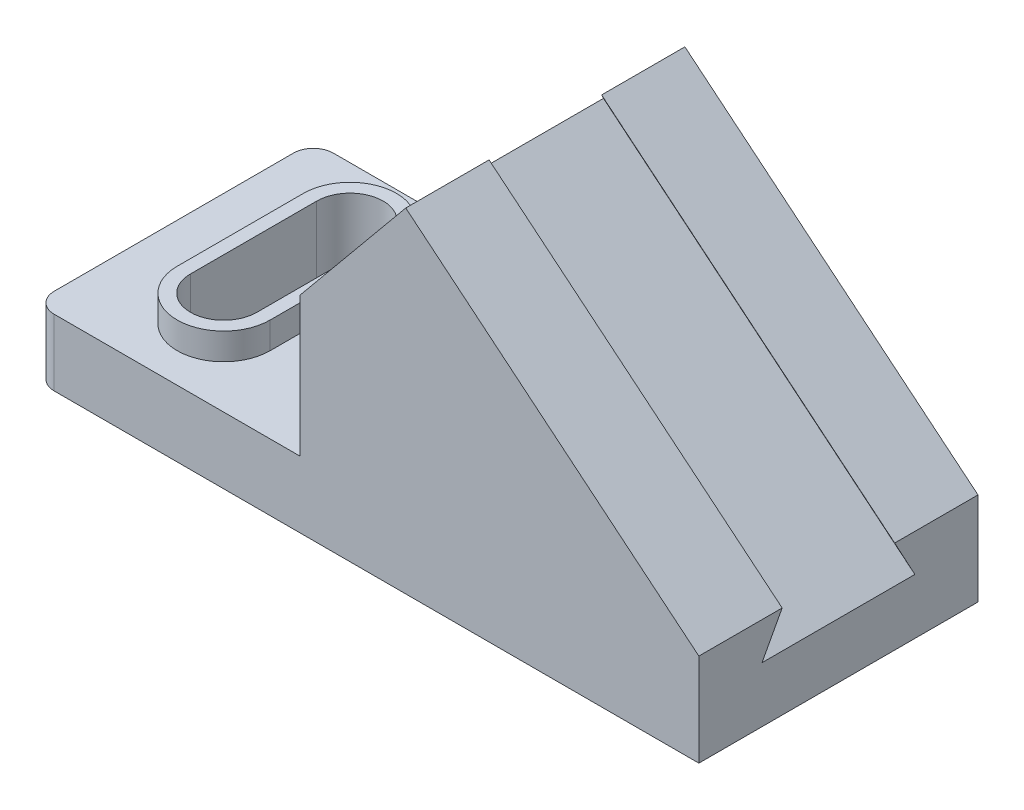
ISO-10303-21;
HEADER;
FILE_DESCRIPTION(('STEP AP214'),'2;1');
FILE_NAME('part.step','',(''),(''),'','','');
FILE_SCHEMA(('AUTOMOTIVE_DESIGN { 1 0 10303 214 1 1 1 1 }'));
ENDSEC;
DATA;
#1=APPLICATION_CONTEXT('core data for automotive mechanical design processes');
#2=APPLICATION_PROTOCOL_DEFINITION('international standard','automotive_design',2000,#1);
#3=PRODUCT_CONTEXT('',#1,'mechanical');
#4=PRODUCT('Part','Part','',(#3));
#5=PRODUCT_RELATED_PRODUCT_CATEGORY('part','',(#4));
#6=PRODUCT_DEFINITION_FORMATION('','',#4);
#7=PRODUCT_DEFINITION_CONTEXT('part definition',#1,'design');
#8=PRODUCT_DEFINITION('design','',#6,#7);
#9=PRODUCT_DEFINITION_SHAPE('','',#8);
#10=(LENGTH_UNIT() NAMED_UNIT(*) SI_UNIT(.MILLI.,.METRE.));
#11=(NAMED_UNIT(*) PLANE_ANGLE_UNIT() SI_UNIT($,.RADIAN.));
#12=(NAMED_UNIT(*) SI_UNIT($,.STERADIAN.) SOLID_ANGLE_UNIT());
#13=UNCERTAINTY_MEASURE_WITH_UNIT(LENGTH_MEASURE(1.E-05),#10,'distance_accuracy_value','');
#14=(GEOMETRIC_REPRESENTATION_CONTEXT(3) GLOBAL_UNCERTAINTY_ASSIGNED_CONTEXT((#13)) GLOBAL_UNIT_ASSIGNED_CONTEXT((#10,
#11,#12)) REPRESENTATION_CONTEXT('',''));
#15=CARTESIAN_POINT('',(0.,0.,0.));
#16=DIRECTION('',(0.,0.,1.));
#17=DIRECTION('',(1.,0.,0.));
#18=AXIS2_PLACEMENT_3D('',#15,#16,#17);
#19=CARTESIAN_POINT('',(-100.,9.99999999999999,21.));
#20=DIRECTION('',(0.,-1.,0.));
#21=DIRECTION('',(0.,0.,-1.));
#22=AXIS2_PLACEMENT_3D('',#19,#20,#21);
#23=PLANE('',#22);
#24=DIRECTION('',(-1.,0.,0.));
#25=VECTOR('',#24,1.);
#26=CARTESIAN_POINT('',(-100.,9.99999999999999,-21.));
#27=LINE('',#26,#25);
#28=CARTESIAN_POINT('',(-60.,9.99999999999999,-21.));
#29=VERTEX_POINT('',#28);
#30=CARTESIAN_POINT('',(-97.,9.99999999999999,-21.));
#31=VERTEX_POINT('',#30);
#32=EDGE_CURVE('E213',#29,#31,#27,.T.);
#33=ORIENTED_EDGE('',*,*,#32,.T.);
#34=CARTESIAN_POINT('',(-97.,9.99999999999999,-18.));
#35=DIRECTION('',(0.,-1.,0.));
#36=DIRECTION('',(0.,0.,-1.));
#37=AXIS2_PLACEMENT_3D('',#34,#35,#36);
#38=CIRCLE('',#37,3.);
#39=CARTESIAN_POINT('',(-100.,9.99999999999999,-18.));
#40=VERTEX_POINT('',#39);
#41=EDGE_CURVE('E50',#31,#40,#38,.F.);
#42=ORIENTED_EDGE('',*,*,#41,.T.);
#43=DIRECTION('',(0.,0.,-1.));
#44=VECTOR('',#43,1.);
#45=CARTESIAN_POINT('',(-100.,9.99999999999999,21.));
#46=LINE('',#45,#44);
#47=CARTESIAN_POINT('',(-100.,9.99999999999999,18.));
#48=VERTEX_POINT('',#47);
#49=EDGE_CURVE('E235',#48,#40,#46,.T.);
#50=ORIENTED_EDGE('',*,*,#49,.F.);
#51=CARTESIAN_POINT('',(-97.,9.99999999999999,18.));
#52=DIRECTION('',(0.,-1.,0.));
#53=DIRECTION('',(0.,0.,-1.));
#54=AXIS2_PLACEMENT_3D('',#51,#52,#53);
#55=CIRCLE('',#54,3.);
#56=CARTESIAN_POINT('',(-97.,9.99999999999999,21.));
#57=VERTEX_POINT('',#56);
#58=EDGE_CURVE('E53',#48,#57,#55,.F.);
#59=ORIENTED_EDGE('',*,*,#58,.T.);
#60=DIRECTION('',(-1.,0.,0.));
#61=VECTOR('',#60,1.);
#62=CARTESIAN_POINT('',(-100.,9.99999999999999,21.));
#63=LINE('',#62,#61);
#64=CARTESIAN_POINT('',(-60.,9.99999999999999,21.));
#65=VERTEX_POINT('',#64);
#66=EDGE_CURVE('E288',#65,#57,#63,.T.);
#67=ORIENTED_EDGE('',*,*,#66,.F.);
#68=DIRECTION('',(0.,0.,-1.));
#69=VECTOR('',#68,1.);
#70=CARTESIAN_POINT('',(-60.,9.99999999999999,21.));
#71=LINE('',#70,#69);
#72=EDGE_CURVE('E232',#65,#29,#71,.T.);
#73=ORIENTED_EDGE('',*,*,#72,.T.);
#74=EDGE_LOOP('',(#33,#42,#50,#59,#67,#73));
#75=FACE_BOUND('',#74,.T.);
#76=CARTESIAN_POINT('',(-83.,9.99999999999999,-9.5));
#77=DIRECTION('',(0.,1.,0.));
#78=DIRECTION('',(0.,0.,1.));
#79=AXIS2_PLACEMENT_3D('',#76,#77,#78);
#80=CIRCLE('',#79,7.00000000000001);
#81=CARTESIAN_POINT('',(-76.,9.99999999999999,-9.5));
#82=VERTEX_POINT('',#81);
#83=CARTESIAN_POINT('',(-90.,9.99999999999999,-9.5));
#84=VERTEX_POINT('',#83);
#85=EDGE_CURVE('E317',#82,#84,#80,.T.);
#86=ORIENTED_EDGE('',*,*,#85,.F.);
#87=DIRECTION('',(0.,0.,-1.));
#88=VECTOR('',#87,1.);
#89=CARTESIAN_POINT('',(-76.,9.99999999999999,-9.5));
#90=LINE('',#89,#88);
#91=CARTESIAN_POINT('',(-76.,9.99999999999999,9.5));
#92=VERTEX_POINT('',#91);
#93=EDGE_CURVE('E306',#92,#82,#90,.T.);
#94=ORIENTED_EDGE('',*,*,#93,.F.);
#95=CARTESIAN_POINT('',(-83.,9.99999999999999,9.5));
#96=DIRECTION('',(0.,1.,0.));
#97=DIRECTION('',(0.,0.,1.));
#98=AXIS2_PLACEMENT_3D('',#95,#96,#97);
#99=CIRCLE('',#98,7.00000000000001);
#100=CARTESIAN_POINT('',(-90.,9.99999999999999,9.5));
#101=VERTEX_POINT('',#100);
#102=EDGE_CURVE('E309',#101,#92,#99,.T.);
#103=ORIENTED_EDGE('',*,*,#102,.F.);
#104=DIRECTION('',(0.,0.,1.));
#105=VECTOR('',#104,1.);
#106=CARTESIAN_POINT('',(-90.,9.99999999999999,-9.5));
#107=LINE('',#106,#105);
#108=EDGE_CURVE('E312',#84,#101,#107,.T.);
#109=ORIENTED_EDGE('',*,*,#108,.F.);
#110=EDGE_LOOP('',(#86,#94,#103,#109));
#111=FACE_BOUND('',#110,.T.);
#112=ADVANCED_FACE('F39',(#75,#111),#23,.F.);
#113=CARTESIAN_POINT('',(0.,22.7360288756917,21.));
#114=DIRECTION('',(-1.,0.,0.));
#115=DIRECTION('',(0.,-1.,0.));
#116=AXIS2_PLACEMENT_3D('',#113,#114,#115);
#117=PLANE('',#116);
#118=DIRECTION('',(0.,0.879756327177352,-0.475424867661984));
#119=VECTOR('',#118,1.);
#120=CARTESIAN_POINT('',(0.,15.5093629916643,7.62731912376527));
#121=LINE('',#120,#119);
#122=CARTESIAN_POINT('',(0.,8.34310868788543,11.5));
#123=VERTEX_POINT('',#122);
#124=CARTESIAN_POINT('',(-1.08873334261842E-13,13.9569215437046,8.4662665085682));
#125=VERTEX_POINT('',#124);
#126=EDGE_CURVE('E344',#123,#125,#121,.T.);
#127=ORIENTED_EDGE('',*,*,#126,.T.);
#128=DIRECTION('',(0.,0.,1.));
#129=VECTOR('',#128,1.);
#130=CARTESIAN_POINT('',(0.,13.9569215437045,21.));
#131=LINE('',#130,#129);
#132=CARTESIAN_POINT('',(0.,13.9569215437045,21.));
#133=VERTEX_POINT('',#132);
#134=EDGE_CURVE('E347',#125,#133,#131,.T.);
#135=ORIENTED_EDGE('',*,*,#134,.T.);
#136=DIRECTION('',(0.,1.,0.));
#137=VECTOR('',#136,1.);
#138=CARTESIAN_POINT('',(0.,22.7360288756917,21.));
#139=LINE('',#138,#137);
#140=CARTESIAN_POINT('',(0.,0.,21.));
#141=VERTEX_POINT('',#140);
#142=EDGE_CURVE('E225',#141,#133,#139,.T.);
#143=ORIENTED_EDGE('',*,*,#142,.F.);
#144=DIRECTION('',(0.,0.,-1.));
#145=VECTOR('',#144,1.);
#146=CARTESIAN_POINT('',(0.,0.,21.));
#147=LINE('',#146,#145);
#148=CARTESIAN_POINT('',(0.,0.,-21.));
#149=VERTEX_POINT('',#148);
#150=EDGE_CURVE('E221',#141,#149,#147,.T.);
#151=ORIENTED_EDGE('',*,*,#150,.T.);
#152=DIRECTION('',(0.,1.,0.));
#153=VECTOR('',#152,1.);
#154=CARTESIAN_POINT('',(0.,22.7360288756917,-21.));
#155=LINE('',#154,#153);
#156=CARTESIAN_POINT('',(0.,13.9569215437045,-21.));
#157=VERTEX_POINT('',#156);
#158=EDGE_CURVE('E214',#149,#157,#155,.T.);
#159=ORIENTED_EDGE('',*,*,#158,.T.);
#160=DIRECTION('',(0.,0.,1.));
#161=VECTOR('',#160,1.);
#162=CARTESIAN_POINT('',(0.,13.9569215437045,21.));
#163=LINE('',#162,#161);
#164=CARTESIAN_POINT('',(0.,13.9569215437045,-8.46626650856829));
#165=VERTEX_POINT('',#164);
#166=EDGE_CURVE('E194',#157,#165,#163,.T.);
#167=ORIENTED_EDGE('',*,*,#166,.T.);
#168=DIRECTION('',(0.,-0.879756327177356,-0.475424867661978));
#169=VECTOR('',#168,1.);
#170=CARTESIAN_POINT('',(0.,33.0762004794339,1.86589067747389));
#171=LINE('',#170,#169);
#172=CARTESIAN_POINT('',(0.,8.34310868788538,-11.5));
#173=VERTEX_POINT('',#172);
#174=EDGE_CURVE('E346',#165,#173,#171,.T.);
#175=ORIENTED_EDGE('',*,*,#174,.T.);
#176=DIRECTION('',(0.,0.,1.));
#177=VECTOR('',#176,1.);
#178=CARTESIAN_POINT('',(0.,8.34310868788541,21.));
#179=LINE('',#178,#177);
#180=EDGE_CURVE('E343',#173,#123,#179,.T.);
#181=ORIENTED_EDGE('',*,*,#180,.T.);
#182=EDGE_LOOP('',(#127,#135,#143,#151,#159,#167,#175,#181));
#183=FACE_BOUND('',#182,.T.);
#184=ADVANCED_FACE('F276',(#183),#117,.F.);
#185=CARTESIAN_POINT('',(-60.,31.,21.));
#186=DIRECTION('',(0.771778566555523,-0.635891377678218,0.));
#187=DIRECTION('',(0.635891377678218,0.771778566555523,0.));
#188=AXIS2_PLACEMENT_3D('',#185,#186,#187);
#189=PLANE('',#188);
#190=DIRECTION('',(0.,0.,-1.));
#191=VECTOR('',#190,1.);
#192=CARTESIAN_POINT('',(-44.1027155580446,50.2944641638881,21.));
#193=LINE('',#192,#191);
#194=CARTESIAN_POINT('',(-44.1027155580446,50.2944641638881,21.));
#195=VERTEX_POINT('',#194);
#196=CARTESIAN_POINT('',(-44.1027155580446,50.2944641638881,8.46626650856824));
#197=VERTEX_POINT('',#196);
#198=EDGE_CURVE('E239',#195,#197,#193,.T.);
#199=ORIENTED_EDGE('',*,*,#198,.T.);
#200=DIRECTION('',(0.520891721970854,0.632203990532382,-0.57357643635105));
#201=VECTOR('',#200,1.);
#202=CARTESIAN_POINT('',(-46.857791537814,46.9506405722212,11.5));
#203=LINE('',#202,#201);
#204=CARTESIAN_POINT('',(-46.857791537814,46.9506405722212,11.5));
#205=VERTEX_POINT('',#204);
#206=EDGE_CURVE('E357',#205,#197,#203,.T.);
#207=ORIENTED_EDGE('',*,*,#206,.F.);
#208=DIRECTION('',(0.,0.,1.));
#209=VECTOR('',#208,1.);
#210=CARTESIAN_POINT('',(-46.857791537814,46.9506405722212,-11.5));
#211=LINE('',#210,#209);
#212=CARTESIAN_POINT('',(-46.857791537814,46.9506405722212,-11.5));
#213=VERTEX_POINT('',#212);
#214=EDGE_CURVE('E364',#213,#205,#211,.T.);
#215=ORIENTED_EDGE('',*,*,#214,.F.);
#216=DIRECTION('',(-0.520891721970857,-0.632203990532386,-0.573576436351044));
#217=VECTOR('',#216,1.);
#218=CARTESIAN_POINT('',(-46.857791537814,46.9506405722212,-11.5));
#219=LINE('',#218,#217);
#220=CARTESIAN_POINT('',(-44.1027155580446,50.2944641638881,-8.46626650856829));
#221=VERTEX_POINT('',#220);
#222=EDGE_CURVE('E206',#221,#213,#219,.T.);
#223=ORIENTED_EDGE('',*,*,#222,.F.);
#224=DIRECTION('',(0.,0.,1.));
#225=VECTOR('',#224,1.);
#226=CARTESIAN_POINT('',(-44.1027155580446,50.2944641638881,-8.46626650856829));
#227=LINE('',#226,#225);
#228=CARTESIAN_POINT('',(-44.1027155580446,50.2944641638881,-21.));
#229=VERTEX_POINT('',#228);
#230=EDGE_CURVE('E188',#229,#221,#227,.T.);
#231=ORIENTED_EDGE('',*,*,#230,.F.);
#232=DIRECTION('',(-0.635891377678218,-0.771778566555523,0.));
#233=VECTOR('',#232,1.);
#234=CARTESIAN_POINT('',(-60.,31.,-21.));
#235=LINE('',#234,#233);
#236=CARTESIAN_POINT('',(-60.,31.,-21.));
#237=VERTEX_POINT('',#236);
#238=EDGE_CURVE('E205',#229,#237,#235,.T.);
#239=ORIENTED_EDGE('',*,*,#238,.T.);
#240=DIRECTION('',(0.,0.,-1.));
#241=VECTOR('',#240,1.);
#242=CARTESIAN_POINT('',(-60.,31.,21.));
#243=LINE('',#242,#241);
#244=CARTESIAN_POINT('',(-60.,31.,21.));
#245=VERTEX_POINT('',#244);
#246=EDGE_CURVE('E238',#245,#237,#243,.T.);
#247=ORIENTED_EDGE('',*,*,#246,.F.);
#248=DIRECTION('',(-0.635891377678218,-0.771778566555523,0.));
#249=VECTOR('',#248,1.);
#250=CARTESIAN_POINT('',(-60.,31.,21.));
#251=LINE('',#250,#249);
#252=EDGE_CURVE('E293',#195,#245,#251,.T.);
#253=ORIENTED_EDGE('',*,*,#252,.F.);
#254=EDGE_LOOP('',(#199,#207,#215,#223,#231,#239,#247,#253));
#255=FACE_BOUND('',#254,.T.);
#256=ADVANCED_FACE('F204',(#255),#189,.F.);
#257=CARTESIAN_POINT('',(-60.,9.99999999999999,21.));
#258=DIRECTION('',(1.,0.,0.));
#259=DIRECTION('',(0.,0.,-1.));
#260=AXIS2_PLACEMENT_3D('',#257,#258,#259);
#261=PLANE('',#260);
#262=DIRECTION('',(0.,-1.,0.));
#263=VECTOR('',#262,1.);
#264=CARTESIAN_POINT('',(-60.,9.99999999999999,-21.));
#265=LINE('',#264,#263);
#266=EDGE_CURVE('E215',#237,#29,#265,.T.);
#267=ORIENTED_EDGE('',*,*,#266,.T.);
#268=ORIENTED_EDGE('',*,*,#72,.F.);
#269=DIRECTION('',(0.,-1.,0.));
#270=VECTOR('',#269,1.);
#271=CARTESIAN_POINT('',(-60.,9.99999999999999,21.));
#272=LINE('',#271,#270);
#273=EDGE_CURVE('E289',#245,#65,#272,.T.);
#274=ORIENTED_EDGE('',*,*,#273,.F.);
#275=ORIENTED_EDGE('',*,*,#246,.T.);
#276=EDGE_LOOP('',(#267,#268,#274,#275));
#277=FACE_BOUND('',#276,.T.);
#278=ADVANCED_FACE('F381',(#277),#261,.F.);
#279=CARTESIAN_POINT('',(-100.,0.,21.));
#280=DIRECTION('',(1.,0.,0.));
#281=DIRECTION('',(0.,0.,-1.));
#282=AXIS2_PLACEMENT_3D('',#279,#280,#281);
#283=PLANE('',#282);
#284=ORIENTED_EDGE('',*,*,#49,.T.);
#285=DIRECTION('',(0.,-1.,0.));
#286=VECTOR('',#285,1.);
#287=CARTESIAN_POINT('',(-100.,0.,-18.));
#288=LINE('',#287,#286);
#289=CARTESIAN_POINT('',(-100.,0.,-18.));
#290=VERTEX_POINT('',#289);
#291=EDGE_CURVE('E260',#40,#290,#288,.T.);
#292=ORIENTED_EDGE('',*,*,#291,.T.);
#293=DIRECTION('',(0.,0.,-1.));
#294=VECTOR('',#293,1.);
#295=CARTESIAN_POINT('',(-100.,0.,21.));
#296=LINE('',#295,#294);
#297=CARTESIAN_POINT('',(-100.,0.,18.));
#298=VERTEX_POINT('',#297);
#299=EDGE_CURVE('E226',#298,#290,#296,.T.);
#300=ORIENTED_EDGE('',*,*,#299,.F.);
#301=DIRECTION('',(0.,-1.,0.));
#302=VECTOR('',#301,1.);
#303=CARTESIAN_POINT('',(-100.,0.,18.));
#304=LINE('',#303,#302);
#305=EDGE_CURVE('E253',#298,#48,#304,.F.);
#306=ORIENTED_EDGE('',*,*,#305,.T.);
#307=EDGE_LOOP('',(#284,#292,#300,#306));
#308=FACE_BOUND('',#307,.T.);
#309=ADVANCED_FACE('F266',(#308),#283,.F.);
#310=CARTESIAN_POINT('',(0.,0.,21.));
#311=DIRECTION('',(0.,1.,0.));
#312=DIRECTION('',(-1.,0.,0.));
#313=AXIS2_PLACEMENT_3D('',#310,#311,#312);
#314=PLANE('',#313);
#315=DIRECTION('',(0.,0.,-1.));
#316=VECTOR('',#315,1.);
#317=CARTESIAN_POINT('',(-78.,0.,20.9999999999999));
#318=LINE('',#317,#316);
#319=CARTESIAN_POINT('',(-78.,0.,9.5));
#320=VERTEX_POINT('',#319);
#321=CARTESIAN_POINT('',(-78.,0.,-9.5));
#322=VERTEX_POINT('',#321);
#323=EDGE_CURVE('E247',#320,#322,#318,.T.);
#324=ORIENTED_EDGE('',*,*,#323,.T.);
#325=CARTESIAN_POINT('',(-83.,0.,-9.5));
#326=DIRECTION('',(0.,1.,0.));
#327=DIRECTION('',(-1.,0.,0.));
#328=AXIS2_PLACEMENT_3D('',#325,#326,#327);
#329=CIRCLE('',#328,5.);
#330=CARTESIAN_POINT('',(-88.,0.,-9.5));
#331=VERTEX_POINT('',#330);
#332=EDGE_CURVE('E196',#322,#331,#329,.T.);
#333=ORIENTED_EDGE('',*,*,#332,.T.);
#334=DIRECTION('',(0.,0.,1.));
#335=VECTOR('',#334,1.);
#336=CARTESIAN_POINT('',(-88.,0.,21.));
#337=LINE('',#336,#335);
#338=CARTESIAN_POINT('',(-88.,0.,9.5));
#339=VERTEX_POINT('',#338);
#340=EDGE_CURVE('E245',#331,#339,#337,.T.);
#341=ORIENTED_EDGE('',*,*,#340,.T.);
#342=CARTESIAN_POINT('',(-83.,0.,9.5));
#343=DIRECTION('',(0.,1.,0.));
#344=DIRECTION('',(-1.,0.,0.));
#345=AXIS2_PLACEMENT_3D('',#342,#343,#344);
#346=CIRCLE('',#345,5.);
#347=EDGE_CURVE('E244',#339,#320,#346,.T.);
#348=ORIENTED_EDGE('',*,*,#347,.T.);
#349=EDGE_LOOP('',(#324,#333,#341,#348));
#350=FACE_BOUND('',#349,.T.);
#351=ORIENTED_EDGE('',*,*,#299,.T.);
#352=CARTESIAN_POINT('',(-97.,0.,-18.));
#353=DIRECTION('',(0.,1.,0.));
#354=DIRECTION('',(-1.,0.,0.));
#355=AXIS2_PLACEMENT_3D('',#352,#353,#354);
#356=CIRCLE('',#355,3.);
#357=CARTESIAN_POINT('',(-97.,0.,-21.));
#358=VERTEX_POINT('',#357);
#359=EDGE_CURVE('E265',#290,#358,#356,.F.);
#360=ORIENTED_EDGE('',*,*,#359,.T.);
#361=DIRECTION('',(1.,0.,0.));
#362=VECTOR('',#361,1.);
#363=CARTESIAN_POINT('',(0.,0.,-21.));
#364=LINE('',#363,#362);
#365=EDGE_CURVE('E224',#358,#149,#364,.T.);
#366=ORIENTED_EDGE('',*,*,#365,.T.);
#367=ORIENTED_EDGE('',*,*,#150,.F.);
#368=DIRECTION('',(1.,0.,0.));
#369=VECTOR('',#368,1.);
#370=CARTESIAN_POINT('',(0.,0.,21.));
#371=LINE('',#370,#369);
#372=CARTESIAN_POINT('',(-97.,0.,21.));
#373=VERTEX_POINT('',#372);
#374=EDGE_CURVE('E230',#373,#141,#371,.T.);
#375=ORIENTED_EDGE('',*,*,#374,.F.);
#376=CARTESIAN_POINT('',(-97.,0.,18.));
#377=DIRECTION('',(0.,1.,0.));
#378=DIRECTION('',(-1.,0.,0.));
#379=AXIS2_PLACEMENT_3D('',#376,#377,#378);
#380=CIRCLE('',#379,3.);
#381=EDGE_CURVE('E258',#373,#298,#380,.F.);
#382=ORIENTED_EDGE('',*,*,#381,.T.);
#383=EDGE_LOOP('',(#351,#360,#366,#367,#375,#382));
#384=FACE_BOUND('',#383,.T.);
#385=ADVANCED_FACE('F273',(#350,#384),#314,.F.);
#386=CARTESIAN_POINT('',(0.,0.,21.));
#387=DIRECTION('',(0.,0.,-1.));
#388=DIRECTION('',(-1.,0.,0.));
#389=AXIS2_PLACEMENT_3D('',#386,#387,#388);
#390=PLANE('',#389);
#391=ORIENTED_EDGE('',*,*,#66,.T.);
#392=DIRECTION('',(0.,-1.,0.));
#393=VECTOR('',#392,1.);
#394=CARTESIAN_POINT('',(-97.,0.,21.));
#395=LINE('',#394,#393);
#396=EDGE_CURVE('E11',#57,#373,#395,.T.);
#397=ORIENTED_EDGE('',*,*,#396,.T.);
#398=ORIENTED_EDGE('',*,*,#374,.T.);
#399=ORIENTED_EDGE('',*,*,#142,.T.);
#400=DIRECTION('',(-0.771778566555523,0.635891377678218,0.));
#401=VECTOR('',#400,1.);
#402=CARTESIAN_POINT('',(6.84960120406021,8.31333083654682,21.));
#403=LINE('',#402,#401);
#404=EDGE_CURVE('E200',#133,#195,#403,.T.);
#405=ORIENTED_EDGE('',*,*,#404,.T.);
#406=ORIENTED_EDGE('',*,*,#252,.T.);
#407=ORIENTED_EDGE('',*,*,#273,.T.);
#408=EDGE_LOOP('',(#391,#397,#398,#399,#405,#406,#407));
#409=FACE_BOUND('',#408,.T.);
#410=ADVANCED_FACE('F379',(#409),#390,.F.);
#411=CARTESIAN_POINT('',(0.,0.,-21.));
#412=DIRECTION('',(0.,0.,-1.));
#413=DIRECTION('',(-1.,0.,0.));
#414=AXIS2_PLACEMENT_3D('',#411,#412,#413);
#415=PLANE('',#414);
#416=ORIENTED_EDGE('',*,*,#365,.F.);
#417=DIRECTION('',(0.,-1.,0.));
#418=VECTOR('',#417,1.);
#419=CARTESIAN_POINT('',(-97.,9.99999999999999,-21.));
#420=LINE('',#419,#418);
#421=EDGE_CURVE('E65',#358,#31,#420,.F.);
#422=ORIENTED_EDGE('',*,*,#421,.T.);
#423=ORIENTED_EDGE('',*,*,#32,.F.);
#424=ORIENTED_EDGE('',*,*,#266,.F.);
#425=ORIENTED_EDGE('',*,*,#238,.F.);
#426=DIRECTION('',(-0.771778566555523,0.635891377678218,0.));
#427=VECTOR('',#426,1.);
#428=CARTESIAN_POINT('',(6.84960120406021,8.31333083654682,-21.));
#429=LINE('',#428,#427);
#430=EDGE_CURVE('E187',#157,#229,#429,.T.);
#431=ORIENTED_EDGE('',*,*,#430,.F.);
#432=ORIENTED_EDGE('',*,*,#158,.F.);
#433=EDGE_LOOP('',(#416,#422,#423,#424,#425,#431,#432));
#434=FACE_BOUND('',#433,.T.);
#435=ADVANCED_FACE('F212',(#434),#415,.T.);
#436=CARTESIAN_POINT('',(-83.,14.,-9.5));
#437=DIRECTION('',(0.,1.,0.));
#438=DIRECTION('',(0.,0.,1.));
#439=AXIS2_PLACEMENT_3D('',#436,#437,#438);
#440=PLANE('',#439);
#441=CARTESIAN_POINT('',(-83.,14.,-9.5));
#442=DIRECTION('',(0.,1.,0.));
#443=DIRECTION('',(0.,0.,1.));
#444=AXIS2_PLACEMENT_3D('',#441,#442,#443);
#445=CIRCLE('',#444,7.00000000000001);
#446=CARTESIAN_POINT('',(-76.,14.,-9.5));
#447=VERTEX_POINT('',#446);
#448=CARTESIAN_POINT('',(-90.,14.,-9.5));
#449=VERTEX_POINT('',#448);
#450=EDGE_CURVE('E307',#447,#449,#445,.T.);
#451=ORIENTED_EDGE('',*,*,#450,.T.);
#452=DIRECTION('',(0.,0.,1.));
#453=VECTOR('',#452,1.);
#454=CARTESIAN_POINT('',(-90.,14.,-9.5));
#455=LINE('',#454,#453);
#456=CARTESIAN_POINT('',(-90.,14.,9.5));
#457=VERTEX_POINT('',#456);
#458=EDGE_CURVE('E324',#449,#457,#455,.T.);
#459=ORIENTED_EDGE('',*,*,#458,.T.);
#460=CARTESIAN_POINT('',(-83.,14.,9.5));
#461=DIRECTION('',(0.,1.,0.));
#462=DIRECTION('',(0.,0.,1.));
#463=AXIS2_PLACEMENT_3D('',#460,#461,#462);
#464=CIRCLE('',#463,7.00000000000001);
#465=CARTESIAN_POINT('',(-76.,14.,9.5));
#466=VERTEX_POINT('',#465);
#467=EDGE_CURVE('E322',#457,#466,#464,.T.);
#468=ORIENTED_EDGE('',*,*,#467,.T.);
#469=DIRECTION('',(0.,0.,-1.));
#470=VECTOR('',#469,1.);
#471=CARTESIAN_POINT('',(-76.,14.,-9.5));
#472=LINE('',#471,#470);
#473=EDGE_CURVE('E304',#466,#447,#472,.T.);
#474=ORIENTED_EDGE('',*,*,#473,.T.);
#475=EDGE_LOOP('',(#451,#459,#468,#474));
#476=FACE_BOUND('',#475,.T.);
#477=DIRECTION('',(0.,0.,1.));
#478=VECTOR('',#477,1.);
#479=CARTESIAN_POINT('',(-88.,14.,-9.5));
#480=LINE('',#479,#478);
#481=CARTESIAN_POINT('',(-88.,14.,-9.5));
#482=VERTEX_POINT('',#481);
#483=CARTESIAN_POINT('',(-88.,14.,9.5));
#484=VERTEX_POINT('',#483);
#485=EDGE_CURVE('E339',#482,#484,#480,.T.);
#486=ORIENTED_EDGE('',*,*,#485,.F.);
#487=CARTESIAN_POINT('',(-83.,14.,-9.5));
#488=DIRECTION('',(0.,1.,0.));
#489=DIRECTION('',(0.,0.,1.));
#490=AXIS2_PLACEMENT_3D('',#487,#488,#489);
#491=CIRCLE('',#490,5.);
#492=CARTESIAN_POINT('',(-78.,14.,-9.5));
#493=VERTEX_POINT('',#492);
#494=EDGE_CURVE('E342',#493,#482,#491,.T.);
#495=ORIENTED_EDGE('',*,*,#494,.F.);
#496=DIRECTION('',(0.,0.,-1.));
#497=VECTOR('',#496,1.);
#498=CARTESIAN_POINT('',(-78.,14.,-9.5));
#499=LINE('',#498,#497);
#500=CARTESIAN_POINT('',(-78.,14.,9.5));
#501=VERTEX_POINT('',#500);
#502=EDGE_CURVE('E335',#501,#493,#499,.T.);
#503=ORIENTED_EDGE('',*,*,#502,.F.);
#504=CARTESIAN_POINT('',(-83.,14.,9.5));
#505=DIRECTION('',(0.,1.,0.));
#506=DIRECTION('',(0.,0.,1.));
#507=AXIS2_PLACEMENT_3D('',#504,#505,#506);
#508=CIRCLE('',#507,5.);
#509=EDGE_CURVE('E337',#484,#501,#508,.T.);
#510=ORIENTED_EDGE('',*,*,#509,.F.);
#511=EDGE_LOOP('',(#486,#495,#503,#510));
#512=FACE_BOUND('',#511,.T.);
#513=ADVANCED_FACE('F461',(#476,#512),#440,.T.);
#514=CARTESIAN_POINT('',(-83.,14.,-9.5));
#515=DIRECTION('',(0.,-1.,0.));
#516=DIRECTION('',(0.,0.,-1.));
#517=AXIS2_PLACEMENT_3D('',#514,#515,#516);
#518=CYLINDRICAL_SURFACE('',#517,7.00000000000001);
#519=ORIENTED_EDGE('',*,*,#85,.T.);
#520=DIRECTION('',(0.,-1.,0.));
#521=VECTOR('',#520,1.);
#522=CARTESIAN_POINT('',(-90.,14.,-9.5));
#523=LINE('',#522,#521);
#524=EDGE_CURVE('E220',#449,#84,#523,.T.);
#525=ORIENTED_EDGE('',*,*,#524,.F.);
#526=ORIENTED_EDGE('',*,*,#450,.F.);
#527=DIRECTION('',(0.,-1.,0.));
#528=VECTOR('',#527,1.);
#529=CARTESIAN_POINT('',(-76.,14.,-9.5));
#530=LINE('',#529,#528);
#531=EDGE_CURVE('E305',#447,#82,#530,.T.);
#532=ORIENTED_EDGE('',*,*,#531,.T.);
#533=EDGE_LOOP('',(#519,#525,#526,#532));
#534=FACE_BOUND('',#533,.T.);
#535=ADVANCED_FACE('F498',(#534),#518,.T.);
#536=CARTESIAN_POINT('',(-90.,14.,-9.5));
#537=DIRECTION('',(1.,0.,0.));
#538=DIRECTION('',(0.,0.,-1.));
#539=AXIS2_PLACEMENT_3D('',#536,#537,#538);
#540=PLANE('',#539);
#541=ORIENTED_EDGE('',*,*,#108,.T.);
#542=DIRECTION('',(0.,-1.,0.));
#543=VECTOR('',#542,1.);
#544=CARTESIAN_POINT('',(-90.,14.,9.5));
#545=LINE('',#544,#543);
#546=EDGE_CURVE('E298',#457,#101,#545,.T.);
#547=ORIENTED_EDGE('',*,*,#546,.F.);
#548=ORIENTED_EDGE('',*,*,#458,.F.);
#549=ORIENTED_EDGE('',*,*,#524,.T.);
#550=EDGE_LOOP('',(#541,#547,#548,#549));
#551=FACE_BOUND('',#550,.T.);
#552=ADVANCED_FACE('F510',(#551),#540,.F.);
#553=CARTESIAN_POINT('',(-83.,14.,9.5));
#554=DIRECTION('',(0.,-1.,0.));
#555=DIRECTION('',(0.,0.,-1.));
#556=AXIS2_PLACEMENT_3D('',#553,#554,#555);
#557=CYLINDRICAL_SURFACE('',#556,7.00000000000001);
#558=ORIENTED_EDGE('',*,*,#102,.T.);
#559=DIRECTION('',(0.,-1.,0.));
#560=VECTOR('',#559,1.);
#561=CARTESIAN_POINT('',(-76.,14.,9.5));
#562=LINE('',#561,#560);
#563=EDGE_CURVE('E299',#466,#92,#562,.T.);
#564=ORIENTED_EDGE('',*,*,#563,.F.);
#565=ORIENTED_EDGE('',*,*,#467,.F.);
#566=ORIENTED_EDGE('',*,*,#546,.T.);
#567=EDGE_LOOP('',(#558,#564,#565,#566));
#568=FACE_BOUND('',#567,.T.);
#569=ADVANCED_FACE('F517',(#568),#557,.T.);
#570=CARTESIAN_POINT('',(-76.,14.,-9.5));
#571=DIRECTION('',(-1.,0.,0.));
#572=DIRECTION('',(0.,0.,1.));
#573=AXIS2_PLACEMENT_3D('',#570,#571,#572);
#574=PLANE('',#573);
#575=ORIENTED_EDGE('',*,*,#93,.T.);
#576=ORIENTED_EDGE('',*,*,#531,.F.);
#577=ORIENTED_EDGE('',*,*,#473,.F.);
#578=ORIENTED_EDGE('',*,*,#563,.T.);
#579=EDGE_LOOP('',(#575,#576,#577,#578));
#580=FACE_BOUND('',#579,.T.);
#581=ADVANCED_FACE('F522',(#580),#574,.F.);
#582=CARTESIAN_POINT('',(-83.,14.,-9.5));
#583=DIRECTION('',(0.,-1.,0.));
#584=DIRECTION('',(0.,0.,-1.));
#585=AXIS2_PLACEMENT_3D('',#582,#583,#584);
#586=CYLINDRICAL_SURFACE('',#585,5.);
#587=DIRECTION('',(0.,-1.,0.));
#588=VECTOR('',#587,1.);
#589=CARTESIAN_POINT('',(-88.,14.,-9.5));
#590=LINE('',#589,#588);
#591=EDGE_CURVE('E316',#482,#331,#590,.T.);
#592=ORIENTED_EDGE('',*,*,#591,.T.);
#593=ORIENTED_EDGE('',*,*,#332,.F.);
#594=DIRECTION('',(0.,-1.,0.));
#595=VECTOR('',#594,1.);
#596=CARTESIAN_POINT('',(-78.,14.,-9.5));
#597=LINE('',#596,#595);
#598=EDGE_CURVE('E334',#493,#322,#597,.T.);
#599=ORIENTED_EDGE('',*,*,#598,.F.);
#600=ORIENTED_EDGE('',*,*,#494,.T.);
#601=EDGE_LOOP('',(#592,#593,#599,#600));
#602=FACE_BOUND('',#601,.T.);
#603=ADVANCED_FACE('F534',(#602),#586,.F.);
#604=CARTESIAN_POINT('',(-88.,14.,-9.5));
#605=DIRECTION('',(1.,0.,0.));
#606=DIRECTION('',(0.,0.,-1.));
#607=AXIS2_PLACEMENT_3D('',#604,#605,#606);
#608=PLANE('',#607);
#609=DIRECTION('',(0.,-1.,0.));
#610=VECTOR('',#609,1.);
#611=CARTESIAN_POINT('',(-88.,14.,9.5));
#612=LINE('',#611,#610);
#613=EDGE_CURVE('E326',#484,#339,#612,.T.);
#614=ORIENTED_EDGE('',*,*,#613,.T.);
#615=ORIENTED_EDGE('',*,*,#340,.F.);
#616=ORIENTED_EDGE('',*,*,#591,.F.);
#617=ORIENTED_EDGE('',*,*,#485,.T.);
#618=EDGE_LOOP('',(#614,#615,#616,#617));
#619=FACE_BOUND('',#618,.T.);
#620=ADVANCED_FACE('F544',(#619),#608,.T.);
#621=CARTESIAN_POINT('',(-83.,14.,9.5));
#622=DIRECTION('',(0.,-1.,0.));
#623=DIRECTION('',(0.,0.,-1.));
#624=AXIS2_PLACEMENT_3D('',#621,#622,#623);
#625=CYLINDRICAL_SURFACE('',#624,5.);
#626=DIRECTION('',(0.,-1.,0.));
#627=VECTOR('',#626,1.);
#628=CARTESIAN_POINT('',(-78.,14.,9.5));
#629=LINE('',#628,#627);
#630=EDGE_CURVE('E327',#501,#320,#629,.T.);
#631=ORIENTED_EDGE('',*,*,#630,.T.);
#632=ORIENTED_EDGE('',*,*,#347,.F.);
#633=ORIENTED_EDGE('',*,*,#613,.F.);
#634=ORIENTED_EDGE('',*,*,#509,.T.);
#635=EDGE_LOOP('',(#631,#632,#633,#634));
#636=FACE_BOUND('',#635,.T.);
#637=ADVANCED_FACE('F551',(#636),#625,.F.);
#638=CARTESIAN_POINT('',(-78.,14.,-9.5));
#639=DIRECTION('',(-1.,0.,0.));
#640=DIRECTION('',(0.,0.,1.));
#641=AXIS2_PLACEMENT_3D('',#638,#639,#640);
#642=PLANE('',#641);
#643=ORIENTED_EDGE('',*,*,#598,.T.);
#644=ORIENTED_EDGE('',*,*,#323,.F.);
#645=ORIENTED_EDGE('',*,*,#630,.F.);
#646=ORIENTED_EDGE('',*,*,#502,.T.);
#647=EDGE_LOOP('',(#643,#644,#645,#646));
#648=FACE_BOUND('',#647,.T.);
#649=ADVANCED_FACE('F417',(#648),#642,.T.);
#650=CARTESIAN_POINT('',(311.247463343949,-248.102958670472,11.5));
#651=DIRECTION('',(0.364732310315032,0.442673999857039,0.819152044288989));
#652=DIRECTION('',(0.,-0.879756327177353,0.475424867661984));
#653=AXIS2_PLACEMENT_3D('',#650,#651,#652);
#654=PLANE('',#653);
#655=DIRECTION('',(-0.771778566555523,0.635891377678218,0.));
#656=VECTOR('',#655,1.);
#657=CARTESIAN_POINT('',(311.247463343949,-248.102958670472,11.5));
#658=LINE('',#657,#656);
#659=EDGE_CURVE('E360',#123,#205,#658,.T.);
#660=ORIENTED_EDGE('',*,*,#659,.T.);
#661=ORIENTED_EDGE('',*,*,#206,.T.);
#662=DIRECTION('',(-0.771778566555523,0.635891377678218,0.));
#663=VECTOR('',#662,1.);
#664=CARTESIAN_POINT('',(314.002539323718,-244.759135078805,8.46626650856824));
#665=LINE('',#664,#663);
#666=EDGE_CURVE('E352',#125,#197,#665,.T.);
#667=ORIENTED_EDGE('',*,*,#666,.F.);
#668=ORIENTED_EDGE('',*,*,#126,.F.);
#669=EDGE_LOOP('',(#660,#661,#667,#668));
#670=FACE_BOUND('',#669,.T.);
#671=ADVANCED_FACE('F376',(#670),#654,.F.);
#672=CARTESIAN_POINT('',(311.247463343949,-248.102958670472,-11.5));
#673=DIRECTION('',(-0.635891377678218,-0.771778566555523,0.));
#674=DIRECTION('',(0.771778566555523,-0.635891377678218,0.));
#675=AXIS2_PLACEMENT_3D('',#672,#673,#674);
#676=PLANE('',#675);
#677=DIRECTION('',(-0.771778566555523,0.635891377678218,0.));
#678=VECTOR('',#677,1.);
#679=CARTESIAN_POINT('',(311.247463343949,-248.102958670472,-11.5));
#680=LINE('',#679,#678);
#681=EDGE_CURVE('E358',#173,#213,#680,.T.);
#682=ORIENTED_EDGE('',*,*,#681,.T.);
#683=ORIENTED_EDGE('',*,*,#214,.T.);
#684=ORIENTED_EDGE('',*,*,#659,.F.);
#685=ORIENTED_EDGE('',*,*,#180,.F.);
#686=EDGE_LOOP('',(#682,#683,#684,#685));
#687=FACE_BOUND('',#686,.T.);
#688=ADVANCED_FACE('F373',(#687),#676,.F.);
#689=CARTESIAN_POINT('',(311.247463343949,-248.102958670472,-11.5));
#690=DIRECTION('',(0.364732310315028,0.442673999857034,-0.819152044288993));
#691=DIRECTION('',(0.,0.879756327177356,0.475424867661978));
#692=AXIS2_PLACEMENT_3D('',#689,#690,#691);
#693=PLANE('',#692);
#694=DIRECTION('',(-0.771778566555523,0.635891377678218,0.));
#695=VECTOR('',#694,1.);
#696=CARTESIAN_POINT('',(314.002539323718,-244.759135078805,-8.46626650856829));
#697=LINE('',#696,#695);
#698=EDGE_CURVE('E355',#165,#221,#697,.T.);
#699=ORIENTED_EDGE('',*,*,#698,.T.);
#700=ORIENTED_EDGE('',*,*,#222,.T.);
#701=ORIENTED_EDGE('',*,*,#681,.F.);
#702=ORIENTED_EDGE('',*,*,#174,.F.);
#703=EDGE_LOOP('',(#699,#700,#701,#702));
#704=FACE_BOUND('',#703,.T.);
#705=ADVANCED_FACE('F367',(#704),#693,.F.);
#706=CARTESIAN_POINT('',(314.002539323718,-244.759135078805,21.));
#707=DIRECTION('',(-0.635891377678218,-0.771778566555523,0.));
#708=DIRECTION('',(0.771778566555523,-0.635891377678218,0.));
#709=AXIS2_PLACEMENT_3D('',#706,#707,#708);
#710=PLANE('',#709);
#711=ORIENTED_EDGE('',*,*,#666,.T.);
#712=ORIENTED_EDGE('',*,*,#198,.F.);
#713=ORIENTED_EDGE('',*,*,#404,.F.);
#714=ORIENTED_EDGE('',*,*,#134,.F.);
#715=EDGE_LOOP('',(#711,#712,#713,#714));
#716=FACE_BOUND('',#715,.T.);
#717=ADVANCED_FACE('F377',(#716),#710,.F.);
#718=CARTESIAN_POINT('',(314.002539323718,-244.759135078805,-8.46626650856829));
#719=DIRECTION('',(-0.635891377678218,-0.771778566555523,0.));
#720=DIRECTION('',(0.771778566555523,-0.635891377678218,0.));
#721=AXIS2_PLACEMENT_3D('',#718,#719,#720);
#722=PLANE('',#721);
#723=ORIENTED_EDGE('',*,*,#430,.T.);
#724=ORIENTED_EDGE('',*,*,#230,.T.);
#725=ORIENTED_EDGE('',*,*,#698,.F.);
#726=ORIENTED_EDGE('',*,*,#166,.F.);
#727=EDGE_LOOP('',(#723,#724,#725,#726));
#728=FACE_BOUND('',#727,.T.);
#729=ADVANCED_FACE('F189',(#728),#722,.F.);
#730=CARTESIAN_POINT('',(-97.,0.,-18.));
#731=DIRECTION('',(0.,1.,0.));
#732=DIRECTION('',(0.,0.,1.));
#733=AXIS2_PLACEMENT_3D('',#730,#731,#732);
#734=CYLINDRICAL_SURFACE('',#733,3.);
#735=ORIENTED_EDGE('',*,*,#41,.F.);
#736=ORIENTED_EDGE('',*,*,#421,.F.);
#737=ORIENTED_EDGE('',*,*,#359,.F.);
#738=ORIENTED_EDGE('',*,*,#291,.F.);
#739=EDGE_LOOP('',(#735,#736,#737,#738));
#740=FACE_BOUND('',#739,.T.);
#741=ADVANCED_FACE('F271',(#740),#734,.T.);
#742=CARTESIAN_POINT('',(-97.,0.,18.));
#743=DIRECTION('',(0.,-1.,0.));
#744=DIRECTION('',(0.,0.,-1.));
#745=AXIS2_PLACEMENT_3D('',#742,#743,#744);
#746=CYLINDRICAL_SURFACE('',#745,3.);
#747=ORIENTED_EDGE('',*,*,#58,.F.);
#748=ORIENTED_EDGE('',*,*,#305,.F.);
#749=ORIENTED_EDGE('',*,*,#381,.F.);
#750=ORIENTED_EDGE('',*,*,#396,.F.);
#751=EDGE_LOOP('',(#747,#748,#749,#750));
#752=FACE_BOUND('',#751,.T.);
#753=ADVANCED_FACE('F41',(#752),#746,.T.);
#754=CLOSED_SHELL('',(#112,#184,#256,#278,#309,#385,#410,#435,#513,#535,#552,#569,#581,#603,
#620,#637,#649,#671,#688,#705,#717,#729,#741,#753));
#755=MANIFOLD_SOLID_BREP('B2',#754);
#756=ADVANCED_BREP_SHAPE_REPRESENTATION('',(#18,#755),#14);
#757=SHAPE_DEFINITION_REPRESENTATION(#9,#756);
ENDSEC;
END-ISO-10303-21;
